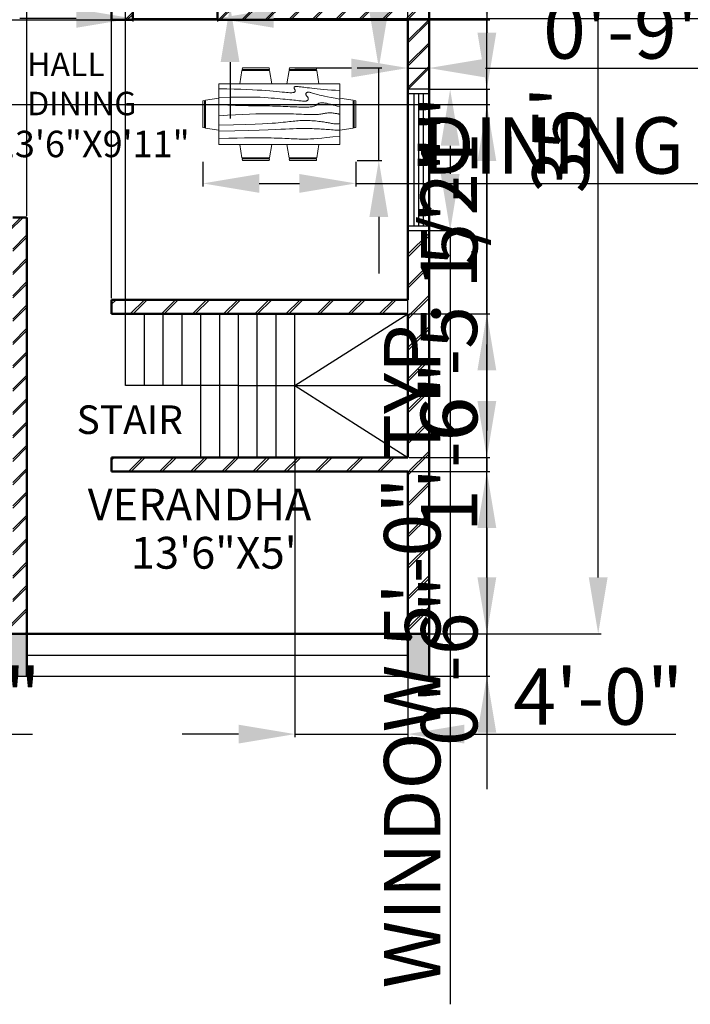
# Model space of a CAD drawing. Units: inches. Extents: x -584 to 444, y 228 to 1001.
# Tile 3 of 5: x -68 to 217, y 228 to 647. Entities that reach past the tile are written whole.
import ezdxf

# ---------------------------------------------------------------- set-up
doc = ezdxf.new("R2010")
doc.units = ezdxf.units.IN
for name, color, linetype, lineweight in [('A-ANNO-DIMS', 2, 'Continuous', 18), ('A-AREA-IDEN', 7, 'Continuous', 25), ('A-FLOR-STRS', 7, 'Continuous', 25), ('A-FURN', 8, 'Continuous', 18), ('A-GLAZ', 4, 'Continuous', 25), ('A-WALL', 7, 'Continuous', 50), ('A-WALL-PATT', 3, 'Continuous', 13)]:
    doc.layers.add(name, color=color, linetype=linetype, lineweight=lineweight)
doc.styles.get("Standard").update_dxf_attribs({"font": 'arial.ttf'})
doc.dimstyles.new('ISO-25', dxfattribs={"dimtxt": 24, "dimasz": 24, "dimexe": 1.25, "dimexo": 0.625, "dimtad": 1, "dimdec": 1, "dimlunit": 3, "dimtxsty": 'Standard', "dimcen": 2.5, "dimadec": 0, "dimazin": 0, "dimtfac": 1, "dimtdec": 1, "dimtmove": 0, "dimatfit": 3, "dimfxl": 1, "dimarcsym": 0})

# ---------------------------------------------------------------- blocks, each defined once
blk = doc.blocks.new('Dining Set - 36 x 72 in.')
for p, q in [((-22.2343, 26.00059), (-23.4847, 17.99762)), ((-22.2304, 26), (-5.7608, 26)), ((-22, 27.5), (-22.1562, 26.50042)), ((-5.8416, 26.5), (-22.1534, 26.5)), ((-22, 27.5), (-6, 27.5)), ((-5.8437, 26.49966), (-6, 27.5)), ((-4.5152, 17.99762), (-5.7655, 25.99926)), ((5.7657, 26.00059), (4.5153, 17.99762)), ((5.7696, 26), (22.2392, 26)), ((6, 27.5), (5.8438, 26.50042)), ((22.1584, 26.5), (5.8466, 26.5)), ((6, 27.5), (22, 27.5)), ((22.1563, 26.49966), (22, 27.5)), ((23.4848, 17.99762), (22.2345, 25.99926)), ((36, 18), (-36, 18)), ((-36, 18), (-36, -18)), ((36, -18), (36, 18)), ((-45.5, 8), (-44.5004, 8.15617)), ((-45.5, 8), (-45.5, -8)), ((-44.5, -8.15843), (-44.5, 8.15338)), ((-44.0006, 8.23428), (-35.9976, 9.48474)), ((-44, 8.23041), (-44, -8.23915)), ((44.0006, 8.23428), (35.9976, 9.48474)), ((44, 8.23041), (44, -8.23915)), ((44.5, -8.15843), (44.5, 8.15338)), ((45.5, 8), (44.5005, 8.15617)), ((45.5, 8), (45.5, -8)), ((-44.4997, -8.15631), (-45.5, -8)), ((-35.9976, -9.48476), (-43.9993, -8.2345)), ((35.9976, -9.48476), (43.9993, -8.2345)), ((44.4997, -8.15631), (45.5, -8)), ((-36, -18), (36, -18)), ((-22.2343, -26.0006), (-23.4847, -17.99762)), ((-4.5152, -17.99762), (-5.7655, -25.99928)), ((5.7657, -26.0006), (4.5153, -17.99762)), ((23.4848, -17.99762), (22.2345, -25.99928)), ((-22.2304, -26), (-5.7608, -26)), ((-22, -27.5), (-22.1562, -26.50044)), ((-5.8416, -26.5), (-22.1534, -26.5)), ((-22, -27.5), (-6, -27.5)), ((-5.8437, -26.49967), (-6, -27.5)), ((5.7696, -26), (22.2392, -26)), ((6, -27.5), (5.8438, -26.50044)), ((22.1584, -26.5), (5.8466, -26.5)), ((6, -27.5), (22, -27.5)), ((22.1563, -26.49967), (22, -27.5))]:
    blk.add_line(p, q)
for points in [[(-36, 15), (-31.1772, 14.97754), (-26.8079, 14.91406), (-22.8538, 14.81543), (-19.276, 14.6875), (-16.0362, 14.53613), (-13.0957, 14.36718), (-10.4159, 14.18652), (-7.9583, 14), (-5.6904, 13.81315), (-3.6035, 13.63021), (-1.6954, 13.45508), (0.0365, 13.29166), (1.5945, 13.14388), (2.9811, 13.01562), (4.1988, 12.9108), (5.25, 12.83333), (6.1393, 12.78613), (6.8802, 12.76823), (7.4883, 12.77767), (7.9792, 12.8125), (8.3685, 12.87077), (8.6719, 12.95052), (8.9049, 13.0498), (9.0833, 13.16666), (9.2205, 13.29899), (9.3216, 13.44401), (9.3895, 13.59879), (9.4271, 13.76041), (9.4373, 13.92594), (9.4232, 14.09245), (9.3875, 14.257), (9.3333, 14.41666), (9.2638, 14.56917), (9.1836, 14.71484), (9.0975, 14.85465), (9.0104, 14.98958), (8.9272, 15.1206), (8.8529, 15.2487), (8.7922, 15.37483), (8.75, 15.5), (8.7305, 15.62467), (8.7344, 15.74739), (8.7617, 15.86621), (8.8125, 15.97916), (8.8867, 16.08431), (8.9844, 16.17968), (9.1055, 16.26334), (9.25, 16.33333), (9.4189, 16.38802), (9.6172, 16.42708), (9.8506, 16.45052), (10.125, 16.45833), (10.4463, 16.45052), (10.8203, 16.42708), (11.2529, 16.38802), (11.75, 16.33333), (12.3184, 16.26318), (12.9694, 16.17838), (13.7151, 16.07991), (14.5677, 15.96875), (15.5395, 15.84586), (16.6426, 15.71224), (17.8893, 15.56884), (19.2917, 15.41666), (20.859, 15.25667), (22.5879, 15.08984), (24.4721, 14.91715), (26.5052, 14.73958), (28.6809, 14.5581), (30.9929, 14.3737), (33.4347, 14.18733), (36, 14)], [(-36, 10), (-28.9766, 10.14274), (-23.1725, 10.20442), (-18.4241, 10.19775), (-14.5677, 10.13541), (-11.4399, 10.03011), (-8.877, 9.89453), (-6.7154, 9.74137), (-4.7917, 9.58333), (-2.9698, 9.43082), (-1.2246, 9.28515), (0.4415, 9.14534), (2.026, 9.01041), (3.5266, 8.87939), (4.9408, 8.7513), (6.266, 8.62516), (7.5, 8.5), (8.6411, 8.37549), (9.6914, 8.2539), (10.6538, 8.13818), (11.5312, 8.03125), (12.3267, 7.93603), (13.043, 7.85547), (13.6831, 7.79248), (14.25, 7.75), (14.7471, 7.7303), (15.1797, 7.73307), (15.5537, 7.75732), (15.875, 7.80208), (16.1494, 7.86637), (16.3828, 7.94922), (16.5811, 8.04964), (16.75, 8.16666), (16.8944, 8.29915), (17.0143, 8.44531), (17.1089, 8.60319), (17.1771, 8.77083), (17.218, 8.94629), (17.2305, 9.1276), (17.2137, 9.31282), (17.1667, 9.5), (17.0895, 9.6875), (16.987, 9.875), (16.8649, 10.0625), (16.7292, 10.25), (16.5856, 10.4375), (16.4401, 10.625), (16.2985, 10.8125), (16.1667, 11), (16.05, 11.18733), (15.9518, 11.3737), (15.8752, 11.5581), (15.8229, 11.73958), (15.798, 11.91715), (15.8034, 12.08984), (15.842, 12.25667), (15.9167, 12.41666), (16.0295, 12.56836), (16.1784, 12.70833), (16.3605, 12.83268), (16.5729, 12.9375), (16.8127, 13.01888), (17.0768, 13.07291), (17.3625, 13.0957), (17.6667, 13.08333), (17.9894, 13.03312), (18.3418, 12.94726), (18.7382, 12.82918), (19.1927, 12.68229), (19.7195, 12.51001), (20.3327, 12.31575), (21.0465, 12.10294), (21.875, 11.875), (22.8357, 11.63354), (23.959, 11.37304), (25.2786, 11.08618), (26.8282, 10.76562), (28.6414, 10.40405), (30.752, 9.99414), (33.1936, 9.52856), (36, 9)], [(-36, 5.5), (-30.7157, 5.3348), (-26.069, 5.20963), (-21.9946, 5.11767), (-18.4271, 5.05208), (-15.3009, 5.00602), (-12.5508, 4.97265), (-10.1112, 4.94515), (-7.9167, 4.91666), (-5.909, 4.88167), (-4.0586, 4.83984), (-2.3429, 4.79215), (-0.7396, 4.73958), (0.7739, 4.6831), (2.22, 4.6237), (3.6213, 4.56233), (5, 4.5), (6.373, 4.43782), (7.7344, 4.3776), (9.0723, 4.32129), (10.375, 4.27083), (11.6309, 4.22819), (12.8281, 4.19531), (13.9551, 4.17415), (15, 4.16666), (15.954, 4.17448), (16.819, 4.19791), (17.6001, 4.23698), (18.3021, 4.29166), (18.9299, 4.36198), (19.4883, 4.44791), (19.9823, 4.54948), (20.4167, 4.66666), (20.7969, 4.79899), (21.1302, 4.94401), (21.4245, 5.09879), (21.6875, 5.26041), (21.9271, 5.42594), (22.1511, 5.59245), (22.3672, 5.757), (22.5834, 5.91666), (22.8065, 6.06868), (23.0404, 6.21093), (23.2879, 6.34147), (23.5521, 6.45833), (23.8358, 6.55957), (24.142, 6.64323), (24.4735, 6.70735), (24.8334, 6.75), (25.2235, 6.76969), (25.642, 6.76692), (26.0858, 6.74267), (26.5521, 6.69791), (27.0379, 6.63362), (27.5404, 6.55078), (28.0565, 6.45036), (28.5834, 6.33333), (29.1242, 6.19987), (29.7071, 6.04687), (30.3661, 5.87044), (31.1354, 5.66666), (32.0493, 5.43164), (33.142, 5.16146), (34.4475, 4.85221), (36, 4.5)], [(-36, -1), (-30.7915, -0.6591), (-26.0195, -0.38216), (-21.6519, -0.16284), (-17.6563, 0.00521), (-14.0005, 0.12833), (-10.6523, 0.21289), (-7.5796, 0.26522), (-4.75, 0.29166), (-2.134, 0.29793), (0.2878, 0.28711), (2.5317, 0.26163), (4.6146, 0.22396), (6.5529, 0.17651), (8.3633, 0.12174), (10.0623, 0.06209), (11.6667, 0), (13.1899, -0.06201), (14.6341, -0.1211), (15.9982, -0.17432), (17.2813, -0.21875), (18.4823, -0.25147), (19.6003, -0.26953), (20.6343, -0.27002), (21.5834, -0.25), (22.4481, -0.20768), (23.2357, -0.14584), (23.9549, -0.06836), (24.6146, 0.02083), (25.2235, 0.11784), (25.7904, 0.21875), (26.3241, 0.31966), (26.8334, 0.41666), (27.3265, 0.50618), (27.8099, 0.58593), (28.2894, 0.65397), (28.7709, 0.70833), (29.2601, 0.74707), (29.763, 0.76823), (30.2855, 0.76985), (30.8334, 0.75), (31.4088, 0.70784), (31.9994, 0.64713), (32.589, 0.57275), (33.1615, 0.48958), (33.7008, 0.4025), (34.1908, 0.3164), (34.6153, 0.23616), (34.9584, 0.16666), (35.2099, 0.11165), (35.3848, 0.07031), (35.504, 0.04069), (35.5886, 0.02083), (35.6594, 0.00879), (35.7377, 0.0026), (35.8442, 0.00032), (36, 0)], [(-36, -6.5), (-27.1843, -6.31267), (-20.084, -6.1263), (-14.469, -5.9419), (-10.1094, -5.76042), (-6.7752, -5.58285), (-4.2363, -5.41016), (-2.2629, -5.24333), (-0.625, -5.08334), (0.8708, -4.93099), (2.2715, -4.78646), (3.5872, -4.64974), (4.8281, -4.52084), (6.0046, -4.39974), (7.127, -4.28646), (8.2053, -4.18099), (9.25, -4.08334), (10.2705, -3.99382), (11.2734, -3.91407), (12.2647, -3.84603), (13.25, -3.79167), (14.2354, -3.75293), (15.2266, -3.73177), (16.2295, -3.73015), (17.25, -3.75), (18.2912, -3.79248), (19.3451, -3.85547), (20.4009, -3.93604), (21.4479, -4.03125), (22.4754, -4.13819), (23.4727, -4.25391), (24.4289, -4.37549), (25.3334, -4.5), (26.1785, -4.62492), (26.9694, -4.74935), (27.7145, -4.87281), (28.4219, -4.99479), (29.1, -5.11483), (29.7572, -5.23242), (30.4016, -5.34709), (31.0417, -5.45834), (31.6837, -5.56437), (32.3262, -5.65821), (32.9658, -5.73153), (33.599, -5.77604), (34.2224, -5.78345), (34.8327, -5.74545), (35.4264, -5.65373), (36, -5.5)], [(-36, -10), (-26.4022, -9.81299), (-18.4675, -9.62891), (-11.9839, -9.45069), (-6.7396, -9.28125), (-2.5226, -9.12354), (0.8789, -8.98047), (3.6769, -8.85498), (6.0833, -8.75), (8.2767, -8.66765), (10.3021, -8.60677), (12.1712, -8.56543), (13.8958, -8.54167), (15.4876, -8.53353), (16.9583, -8.53907), (18.3197, -8.55632), (19.5834, -8.58334), (20.7616, -8.61841), (21.8685, -8.66081), (22.9188, -8.71004), (23.9271, -8.76563), (24.9081, -8.82707), (25.8763, -8.89388), (26.8465, -8.96558), (27.8334, -9.04167), (28.8474, -9.12118), (29.8828, -9.20117), (30.93, -9.27824), (31.9792, -9.34896), (33.0205, -9.40991), (34.0443, -9.45768), (35.0407, -9.48885), (36, -9.5)], [(-36, -14.5), (-30.0881, -14.33513), (-25.0332, -14.21224), (-20.7312, -14.12647), (-17.0781, -14.07292), (-13.97, -14.04671), (-11.3027, -14.04297), (-8.9724, -14.05681), (-6.875, -14.08334), (-4.9224, -14.11833), (-3.0905, -14.16016), (-1.3709, -14.20785), (0.2448, -14.26042), (1.7647, -14.3169), (3.1973, -14.3763), (4.5507, -14.43767), (5.8333, -14.5), (7.0554, -14.5621), (8.235, -14.62175), (9.3922, -14.67652), (10.5469, -14.72396), (11.7192, -14.76164), (12.929, -14.78711), (14.1965, -14.79794), (15.5417, -14.79167), (16.9933, -14.76424), (18.6152, -14.70508), (20.4804, -14.60197), (22.6615, -14.44271), (25.2312, -14.21509), (28.2624, -13.9069), (31.8277, -13.50594), (36, -13)]]:
    blk.add_lwpolyline(points)
blk = doc.blocks.new('*D7')
at = {"layer": 'A-ANNO-DIMS', "color": 0, "lineweight": -2, "transparency": 16777216}
for p, q in [((106.48, 805.54), (179.05, 805.54)), ((177.8, 409.54), (177.8, 781.54)), ((106.48, 385.54), (179.05, 385.54))]:
    blk.add_line(p, q, dxfattribs=at)
at = {"layer": 'A-ANNO-DIMS', "color": 0, "transparency": 16777216}
for points in [[(173.8, 781.54), (181.8, 781.54), (177.8, 805.54)], [(173.8, 409.54), (181.8, 409.54), (177.8, 385.54)]]:
    blk.add_solid(points, dxfattribs=at)
at = {"layer": 'Defpoints', "color": 0, "transparency": 16777216}
for p in [(105.86, 805.54), (177.8, 805.54), (105.86, 385.54)]:
    blk.add_point(p, dxfattribs=at)
at = {"layer": 'A-ANNO-DIMS', "color": 0, "transparency": 16777216, "insert": (164.91, 595.54), "char_height": 24, "attachment_point": 5, "rotation": 90}
blk.add_mtext("35'", dxfattribs=at)
blk = doc.blocks.new('WIN-60IN')
for p, q in [((60, 9), (0, 9)), ((0, 9), (0, 0)), ((2, 9), (2, 0)), ((58, 0), (58, 9)), ((60, 0), (60, 9)), ((2, 6.5), (58, 6.5)), ((2, 4.5), (58, 4.5)), ((0, 0), (60, 0)), ((2, 2.5), (58, 2.5))]:
    blk.add_line(p, q)
blk = doc.blocks.new('*D11')
at = {"layer": 'A-ANNO-DIMS', "color": 0, "lineweight": -2, "transparency": 16777216}
for p, q in [((106.48, 617.04), (116.11, 617.04)), ((114.86, 593.04), (114.86, 581.04)), ((106.48, 557.04), (116.11, 557.04)), ((114.86, 557.04), (114.86, 228.09))]:
    blk.add_line(p, q, dxfattribs=at)
at = {"layer": 'A-ANNO-DIMS', "color": 0, "transparency": 16777216}
for points in [[(110.86, 593.04), (118.86, 593.04), (114.86, 617.04)], [(110.86, 581.04), (118.86, 581.04), (114.86, 557.04)]]:
    blk.add_solid(points, dxfattribs=at)
at = {"layer": 'Defpoints', "color": 0, "transparency": 16777216}
for p in [(105.86, 617.04), (105.86, 557.04), (114.86, 557.04)]:
    blk.add_point(p, dxfattribs=at)
at = {"layer": 'A-ANNO-DIMS', "color": 0, "transparency": 16777216, "insert": (101.81, 380.56), "char_height": 24, "attachment_point": 5, "rotation": 90}
blk.add_mtext('WINDOW 5\'-0" TYP.', dxfattribs=at)
blk = doc.blocks.new('*D12')
at = {"layer": 'A-ANNO-DIMS', "color": 0, "lineweight": -2, "transparency": 16777216}
for p, q in [((72.86, 626.04), (48.86, 626.04)), ((96.86, 617.66), (96.86, 627.29)), ((96.86, 626.04), (105.86, 626.04)), ((105.86, 617.66), (105.86, 627.29)), ((129.86, 626.04), (301.4, 626.04))]:
    blk.add_line(p, q, dxfattribs=at)
at = {"layer": 'A-ANNO-DIMS', "color": 0, "transparency": 16777216}
for points in [[(72.86, 630.04), (72.86, 622.04), (96.86, 626.04)], [(129.86, 630.04), (129.86, 622.04), (105.86, 626.04)]]:
    blk.add_solid(points, dxfattribs=at)
at = {"layer": 'Defpoints', "color": 0, "transparency": 16777216}
for p in [(105.86, 626.04), (96.86, 617.04), (105.86, 617.04)]:
    blk.add_point(p, dxfattribs=at)
at = {"layer": 'A-ANNO-DIMS', "color": 0, "transparency": 16777216, "insert": (227.63, 638.92), "char_height": 24, "attachment_point": 5}
blk.add_mtext('0\'-9" TYP.', dxfattribs=at)
blk = doc.blocks.new('*D17')
at = {"layer": 'A-ANNO-DIMS', "color": 0, "lineweight": -2, "transparency": 16777216}
for p, q in [((-20.14, 651.91), (-20.14, 645.89)), ((15.86, 651.91), (15.86, 645.89)), ((-44.14, 647.14), (-68.14, 647.14)), ((-20.14, 647.14), (15.86, 647.14)), ((39.86, 647.14), (444.11, 647.14))]:
    blk.add_line(p, q, dxfattribs=at)
at = {"layer": 'A-ANNO-DIMS', "color": 0, "transparency": 16777216}
for points in [[(-44.14, 651.14), (-44.14, 643.14), (-20.14, 647.14)], [(39.86, 651.14), (39.86, 643.14), (15.86, 647.14)]]:
    blk.add_solid(points, dxfattribs=at)
at = {"layer": 'Defpoints', "color": 0, "transparency": 16777216}
for p in [(-20.14, 652.54), (15.86, 652.54), (15.86, 647.14)]:
    blk.add_point(p, dxfattribs=at)
at = {"layer": 'A-ANNO-DIMS', "color": 0, "transparency": 16777216, "insert": (253.99, 660.19), "char_height": 24, "attachment_point": 5}
blk.add_mtext('SWING DOOR 3\'-0" TYP.', dxfattribs=at)
blk = doc.blocks.new('*D18')
at = {"layer": 'A-ANNO-DIMS', "color": 0, "lineweight": -2, "transparency": 16777216}
for p, q in [((21.26, 712.54), (21.26, 884.06)), ((16.48, 688.54), (22.51, 688.54)), ((21.26, 652.54), (21.26, 688.54)), ((16.48, 652.54), (22.51, 652.54)), ((21.26, 628.54), (21.26, 604.54))]:
    blk.add_line(p, q, dxfattribs=at)
at = {"layer": 'A-ANNO-DIMS', "color": 0, "transparency": 16777216}
for points in [[(17.26, 712.54), (25.26, 712.54), (21.26, 688.54)], [(17.26, 628.54), (25.26, 628.54), (21.26, 652.54)]]:
    blk.add_solid(points, dxfattribs=at)
at = {"layer": 'Defpoints', "color": 0, "transparency": 16777216}
for p in [(15.86, 688.54), (21.26, 688.54), (15.86, 652.54)]:
    blk.add_point(p, dxfattribs=at)
at = {"layer": 'A-ANNO-DIMS', "color": 0, "transparency": 16777216, "insert": (8.37, 810.3), "char_height": 24, "attachment_point": 5, "rotation": 90}
blk.add_mtext('3\'-0" TYP.', dxfattribs=at)
blk = doc.blocks.new('*D25')
at = {"layer": 'A-ANNO-DIMS', "color": 0, "lineweight": -2, "transparency": 16777216}
for p, q in [((9.69, 586.14), (9.69, 575.76)), ((74.75, 586.14), (74.75, 575.76)), ((33.69, 577.01), (50.75, 577.01)), ((74.75, 577.01), (363.79, 577.01))]:
    blk.add_line(p, q, dxfattribs=at)
at = {"layer": 'A-ANNO-DIMS', "color": 0, "transparency": 16777216}
for points in [[(33.69, 581.01), (33.69, 573.01), (9.69, 577.01)], [(50.75, 581.01), (50.75, 573.01), (74.75, 577.01)]]:
    blk.add_solid(points, dxfattribs=at)
at = {"layer": 'Defpoints', "color": 0, "transparency": 16777216}
for p in [(9.69, 586.77), (74.75, 586.77), (74.75, 577.01)]:
    blk.add_point(p, dxfattribs=at)
at = {"layer": 'A-ANNO-DIMS', "color": 0, "transparency": 16777216, "insert": (231.27, 590.04), "char_height": 24, "attachment_point": 5}
blk.add_mtext('DINING SET 5\'-5"', dxfattribs=at)
blk = doc.blocks.new('*D26')
at = {"layer": 'A-ANNO-DIMS', "color": 0, "lineweight": -2, "transparency": 16777216}
for p, q in [((84.51, 650.09), (84.51, 795.05)), ((75.37, 626.09), (85.76, 626.09)), ((84.51, 586.77), (84.51, 626.09)), ((75.37, 586.77), (85.76, 586.77)), ((84.51, 562.77), (84.51, 538.77))]:
    blk.add_line(p, q, dxfattribs=at)
at = {"layer": 'A-ANNO-DIMS', "color": 0, "transparency": 16777216}
for points in [[(80.51, 650.09), (88.51, 650.09), (84.51, 626.09)], [(80.51, 562.77), (88.51, 562.77), (84.51, 586.77)]]:
    blk.add_solid(points, dxfattribs=at)
at = {"layer": 'Defpoints', "color": 0, "transparency": 16777216}
for p in [(74.75, 626.09), (84.51, 626.09), (74.75, 586.77)]:
    blk.add_point(p, dxfattribs=at)
at = {"layer": 'A-ANNO-DIMS', "color": 0, "transparency": 16777216, "insert": (71.46, 734.57), "char_height": 24, "attachment_point": 5, "rotation": 90}
blk.add_mtext('3\'-3 1/2"', dxfattribs=at)
blk = doc.blocks.new('*D27')
at = {"layer": 'A-ANNO-DIMS', "color": 0, "lineweight": -2, "transparency": 16777216}
for p, q in [((130.46, 409.54), (130.46, 496.33)), ((106.48, 385.54), (131.71, 385.54)), ((130.46, 367.54), (130.46, 385.54)), ((106.48, 367.54), (131.71, 367.54)), ((130.46, 343.54), (130.46, 319.54))]:
    blk.add_line(p, q, dxfattribs=at)
at = {"layer": 'A-ANNO-DIMS', "color": 0, "transparency": 16777216}
for points in [[(126.46, 409.54), (134.46, 409.54), (130.46, 385.54)], [(126.46, 343.54), (134.46, 343.54), (130.46, 367.54)]]:
    blk.add_solid(points, dxfattribs=at)
at = {"layer": 'Defpoints', "color": 0, "transparency": 16777216}
for p in [(105.86, 385.54), (130.46, 385.54), (105.86, 367.54)]:
    blk.add_point(p, dxfattribs=at)
at = {"layer": 'A-ANNO-DIMS', "color": 0, "transparency": 16777216, "insert": (117.58, 464.93), "char_height": 24, "attachment_point": 5, "rotation": 90}
blk.add_mtext('1\'-6"', dxfattribs=at)
blk = doc.blocks.new('*D29')
at = {"layer": 'A-ANNO-DIMS', "color": 0, "lineweight": -2, "transparency": 16777216}
for p, q in [((-209.14, 795.91), (-209.14, 341.69)), ((-176.14, 795.91), (-176.14, 341.69)), ((-233.14, 342.94), (-257.14, 342.94)), ((-209.14, 342.94), (-176.14, 342.94)), ((-152.14, 342.94), (-62.69, 342.94))]:
    blk.add_line(p, q, dxfattribs=at)
at = {"layer": 'A-ANNO-DIMS', "color": 0, "transparency": 16777216}
for points in [[(-233.14, 346.94), (-233.14, 338.94), (-209.14, 342.94)], [(-152.14, 346.94), (-152.14, 338.94), (-176.14, 342.94)]]:
    blk.add_solid(points, dxfattribs=at)
at = {"layer": 'Defpoints', "color": 0, "transparency": 16777216}
for p in [(-209.14, 796.54), (-176.14, 796.54), (-176.14, 342.94)]:
    blk.add_point(p, dxfattribs=at)
at = {"layer": 'A-ANNO-DIMS', "color": 0, "transparency": 16777216, "insert": (-95.41, 355.82), "char_height": 24, "attachment_point": 5}
blk.add_mtext('2\'-9"', dxfattribs=at)
blk = doc.blocks.new('*D32')
at = {"layer": 'A-ANNO-DIMS', "color": 0, "lineweight": -2, "transparency": 16777216}
for p, q in [((106.48, 694.54), (131.71, 694.54)), ((130.46, 670.54), (130.46, 641.04)), ((106.48, 617.04), (131.71, 617.04)), ((130.46, 617.04), (130.46, 471.93))]:
    blk.add_line(p, q, dxfattribs=at)
at = {"layer": 'A-ANNO-DIMS', "color": 0, "transparency": 16777216}
for points in [[(126.46, 670.54), (134.46, 670.54), (130.46, 694.54)], [(126.46, 641.04), (134.46, 641.04), (130.46, 617.04)]]:
    blk.add_solid(points, dxfattribs=at)
at = {"layer": 'Defpoints', "color": 0, "transparency": 16777216}
for p in [(105.86, 694.54), (105.86, 617.04), (130.46, 617.04)]:
    blk.add_point(p, dxfattribs=at)
at = {"layer": 'A-ANNO-DIMS', "color": 0, "transparency": 16777216, "insert": (117.42, 532.49), "char_height": 24, "attachment_point": 5, "rotation": 90}
blk.add_mtext('6\'-5 1/2"', dxfattribs=at)
blk = doc.blocks.new('*D35')
at = {"layer": 'A-ANNO-DIMS', "color": 0, "lineweight": -2, "transparency": 16777216}
for p, q in [((130.46, 484.54), (130.46, 508.54)), ((97.48, 460.54), (131.71, 460.54)), ((130.46, 460.54), (130.46, 454.54)), ((97.48, 454.54), (131.71, 454.54)), ((130.46, 430.54), (130.46, 341.49))]:
    blk.add_line(p, q, dxfattribs=at)
at = {"layer": 'A-ANNO-DIMS', "color": 0, "transparency": 16777216}
for points in [[(126.46, 484.54), (134.46, 484.54), (130.46, 460.54)], [(126.46, 430.54), (134.46, 430.54), (130.46, 454.54)]]:
    blk.add_solid(points, dxfattribs=at)
at = {"layer": 'Defpoints', "color": 0, "transparency": 16777216}
for p in [(96.86, 460.54), (96.86, 454.54), (130.46, 454.54)]:
    blk.add_point(p, dxfattribs=at)
at = {"layer": 'A-ANNO-DIMS', "color": 0, "transparency": 16777216, "insert": (117.58, 374.01), "char_height": 24, "attachment_point": 5, "rotation": 90}
blk.add_mtext('0\'-6"', dxfattribs=at)
blk = doc.blocks.new('*D36')
at = {"layer": 'A-ANNO-DIMS', "color": 0, "lineweight": -2, "transparency": 16777216}
for p, q in [((-23.14, 522.16), (-23.14, 831.39)), ((0.86, 830.14), (72.86, 830.14)), ((96.86, 522.16), (96.86, 831.39))]:
    blk.add_line(p, q, dxfattribs=at)
at = {"layer": 'A-ANNO-DIMS', "color": 0, "transparency": 16777216}
for points in [[(0.86, 834.14), (0.86, 826.14), (-23.14, 830.14)], [(72.86, 834.14), (72.86, 826.14), (96.86, 830.14)]]:
    blk.add_solid(points, dxfattribs=at)
at = {"layer": 'Defpoints', "color": 0, "transparency": 16777216}
for p in [(96.86, 830.14), (-23.14, 521.54), (96.86, 521.54)]:
    blk.add_point(p, dxfattribs=at)
at = {"layer": 'A-ANNO-DIMS', "color": 0, "transparency": 16777216, "insert": (36.86, 843.02), "char_height": 24, "attachment_point": 5}
blk.add_mtext('10\'-0"', dxfattribs=at)
blk = doc.blocks.new('*D37')
at = {"layer": 'A-ANNO-DIMS', "color": 0, "lineweight": -2, "transparency": 16777216}
for p, q in [((48.86, 459.91), (48.86, 341.69)), ((96.86, 453.91), (96.86, 341.69)), ((24.86, 342.94), (0.86, 342.94)), ((48.86, 342.94), (96.86, 342.94)), ((120.86, 342.94), (210.87, 342.94))]:
    blk.add_line(p, q, dxfattribs=at)
at = {"layer": 'A-ANNO-DIMS', "color": 0, "transparency": 16777216}
for points in [[(24.86, 346.94), (24.86, 338.94), (48.86, 342.94)], [(120.86, 346.94), (120.86, 338.94), (96.86, 342.94)]]:
    blk.add_solid(points, dxfattribs=at)
at = {"layer": 'Defpoints', "color": 0, "transparency": 16777216}
for p in [(48.86, 460.54), (96.86, 454.54), (96.86, 342.94)]:
    blk.add_point(p, dxfattribs=at)
at = {"layer": 'A-ANNO-DIMS', "color": 0, "transparency": 16777216, "insert": (177.86, 355.82), "char_height": 24, "attachment_point": 5}
blk.add_mtext('4\'-0"', dxfattribs=at)
blk = doc.blocks.new('*D38')
at = {"layer": 'A-ANNO-DIMS', "color": 0, "lineweight": -2, "transparency": 16777216}
for p, q in [((130.46, 521.54), (130.46, 610.59)), ((97.48, 521.54), (131.71, 521.54)), ((130.46, 484.54), (130.46, 497.54)), ((97.48, 460.54), (131.71, 460.54))]:
    blk.add_line(p, q, dxfattribs=at)
at = {"layer": 'A-ANNO-DIMS', "color": 0, "transparency": 16777216}
for points in [[(126.46, 497.54), (134.46, 497.54), (130.46, 521.54)], [(126.46, 484.54), (134.46, 484.54), (130.46, 460.54)]]:
    blk.add_solid(points, dxfattribs=at)
at = {"layer": 'Defpoints', "color": 0, "transparency": 16777216}
for p in [(96.86, 521.54), (130.46, 521.54), (96.86, 460.54)]:
    blk.add_point(p, dxfattribs=at)
at = {"layer": 'A-ANNO-DIMS', "color": 0, "transparency": 16777216, "insert": (117.58, 578.06), "char_height": 24, "attachment_point": 5, "rotation": 90}
blk.add_mtext('5\'-1"', dxfattribs=at)
blk = doc.blocks.new('*D40')
at = {"layer": 'A-ANNO-DIMS', "color": 0, "lineweight": -2, "transparency": 16777216}
for p, q in [((130.46, 670.54), (130.46, 759.57)), ((-76.52, 646.54), (131.71, 646.54)), ((130.46, 610.54), (130.46, 646.54)), ((-116.52, 610.54), (131.71, 610.54)), ((130.46, 586.54), (130.46, 562.54))]:
    blk.add_line(p, q, dxfattribs=at)
at = {"layer": 'A-ANNO-DIMS', "color": 0, "transparency": 16777216}
for points in [[(126.46, 670.54), (134.46, 670.54), (130.46, 646.54)], [(126.46, 586.54), (134.46, 586.54), (130.46, 610.54)]]:
    blk.add_solid(points, dxfattribs=at)
at = {"layer": 'Defpoints', "color": 0, "transparency": 16777216}
for p in [(-77.14, 646.54), (130.46, 646.54), (-117.14, 610.54)]:
    blk.add_point(p, dxfattribs=at)
at = {"layer": 'A-ANNO-DIMS', "color": 0, "transparency": 16777216, "insert": (117.57, 727.05), "char_height": 24, "attachment_point": 5, "rotation": 90}
blk.add_mtext('3\'-0"', dxfattribs=at)
blk = doc.blocks.new('*D41')
at = {"layer": 'A-ANNO-DIMS', "color": 0, "lineweight": -2, "transparency": 16777216}
for p, q in [((-89.14, 830.14), (-113.14, 830.14)), ((-65.14, 563.16), (-65.14, 831.39)), ((-65.14, 830.14), (-29.14, 830.14)), ((-29.14, 528.16), (-29.14, 831.39)), ((-5.14, 830.14), (83.89, 830.14))]:
    blk.add_line(p, q, dxfattribs=at)
at = {"layer": 'A-ANNO-DIMS', "color": 0, "transparency": 16777216}
for points in [[(-89.14, 834.14), (-89.14, 826.14), (-65.14, 830.14)], [(-5.14, 834.14), (-5.14, 826.14), (-29.14, 830.14)]]:
    blk.add_solid(points, dxfattribs=at)
at = {"layer": 'Defpoints', "color": 0, "transparency": 16777216}
for p in [(-29.14, 830.14), (-65.14, 562.54), (-29.14, 527.54)]:
    blk.add_point(p, dxfattribs=at)
at = {"layer": 'A-ANNO-DIMS', "color": 0, "transparency": 16777216, "insert": (51.37, 843.02), "char_height": 24, "attachment_point": 5}
blk.add_mtext('3\'-0"', dxfattribs=at)

msp = doc.modelspace()

# ---------------------------------------------------------------- hatches: boundary and pattern name
at = {"layer": 'A-WALL-PATT'}
h = msp.add_hatch(dxfattribs=at)
h.set_pattern_fill('JIS_LC_8A', color=256, scale=0.9)
h.set_pattern_definition([(45, (105.857, 805.537), (-4.96389, 4.96389), []), (45, (106.757, 805.537), (-4.96389, 4.96389), [])])
h.paths.add_polyline_path([(105.86, 694.54), (96.86, 694.54), (96.86, 652.54), (15.86, 652.54), (15.86, 646.54), (96.86, 646.54), (96.86, 617.04), (105.86, 617.04)])
h.paths.add_polyline_path([(-77.14, 655.54), (-83.14, 655.54), (-83.14, 652.54), (-209.14, 652.54), (-209.14, 796.54), (-176.14, 796.54), (-176.14, 805.54), (-218.14, 805.54), (-218.14, 610.54), (-209.14, 610.54), (-209.14, 646.54), (-77.14, 646.54)])
h.paths.add_polyline_path([(-209.14, 598.54), (-218.14, 598.54), (-218.14, 505.54), (-209.14, 505.54), (-209.14, 556.54), (-111.14, 556.54), (-110.14, 556.54), (-110.14, 562.54), (-111.14, 562.54), (-111.14, 610.54), (-117.14, 610.54), (-117.14, 562.54), (-209.14, 562.54)])
h.paths.add_polyline_path([(-59.14, 805.54), (-116.14, 805.54), (-116.14, 796.54), (-83.14, 796.54), (-83.14, 691.54), (-77.14, 691.54), (-77.14, 796.54), (-59.14, 796.54)])
h.paths.add_polyline_path([(105.86, 805.54), (-47.14, 805.54), (-47.14, 796.54), (-29.14, 796.54), (-29.14, 712.54), (-47.14, 712.54), (-47.14, 706.54), (-29.14, 706.54), (-29.14, 646.54), (-20.14, 646.54), (-20.14, 652.54), (-23.14, 652.54), (-23.14, 796.54), (96.86, 796.54), (96.86, 754.54), (105.86, 754.54)])
h.paths.add_polyline_path([(-65.14, 385.54), (-65.14, 562.54), (-71.14, 562.54), (-74.14, 562.54), (-74.14, 556.54), (-71.14, 556.54), (-71.14, 394.54), (-209.14, 394.54), (-209.14, 445.54), (-218.14, 445.54), (-218.14, 385.54)])
h = msp.add_hatch(dxfattribs=at)
h.set_pattern_fill('JIS_LC_8A', color=256, scale=1.2)
h.paths.add_polyline_path([(105.86, 557.04), (96.86, 557.04), (96.86, 527.54), (-29.14, 527.54), (-29.14, 521.54), (96.86, 521.54), (96.86, 460.54), (-29.14, 460.54), (-29.14, 454.54), (96.86, 454.54), (96.86, 394.54), (96.86, 385.54), (105.86, 385.54)])
h = msp.add_hatch(dxfattribs=at)
h.set_pattern_fill('BRICK', color=256, scale=0.2)
h.paths.add_polyline_path([(-65.14, 385.54), (-74.14, 385.54), (-74.14, 367.54), (-65.14, 367.54)])
h.paths.add_polyline_path([(105.86, 385.54), (96.86, 385.54), (96.86, 367.54), (105.86, 367.54)])

# ---------------------------------------------------------------- linework, layer by layer
at = {"layer": 'A-FLOR-STRS'}
for p, q in [((-23.14, 491.04), (-23.14, 521.54)), ((-15.14, 491.04), (-15.14, 521.54)), ((-7.14, 491.04), (-7.14, 521.54)), ((0.86, 491.04), (0.86, 521.54)), ((8.86, 460.54), (8.86, 521.54)), ((16.86, 460.54), (16.86, 521.54)), ((24.86, 460.54), (24.86, 521.54)), ((32.86, 460.54), (32.86, 521.54)), ((40.86, 460.54), (40.86, 521.54)), ((48.86, 460.54), (48.86, 521.54)), ((48.86, 491.04), (96.86, 521.54)), ((24.86, 491.04), (-23.14, 491.04)), ((24.86, 491.04), (96.86, 491.04)), ((48.86, 491.04), (96.86, 460.54)), ((-65.14, 376.54), (96.86, 376.54)), ((-74.14, 367.54), (105.86, 367.54))]:
    msp.add_line(p, q, dxfattribs=at)
at = {"layer": 'A-WALL'}
for p, q in [((105.86, 385.54), (105.86, 805.54)), ((-29.14, 706.54), (-29.14, 646.54)), ((-20.14, 652.54), (-20.14, 646.54)), ((15.86, 652.54), (15.86, 646.54)), ((-20.14, 646.54), (-29.14, 646.54)), ((96.86, 646.54), (15.86, 646.54)), ((96.86, 527.54), (96.86, 646.54)), ((-71.14, 562.54), (-65.14, 562.54)), ((-65.14, 556.54), (-65.14, 562.54)), ((-65.14, 556.54), (-65.14, 394.54)), ((96.86, 527.54), (-29.14, 527.54)), ((-29.14, 527.54), (-29.14, 521.54)), ((96.86, 521.54), (-29.14, 521.54)), ((96.86, 460.54), (96.86, 521.54)), ((-29.14, 460.54), (-29.14, 454.54)), ((-29.14, 460.54), (96.86, 460.54)), ((-29.14, 454.54), (96.86, 454.54)), ((96.86, 394.54), (96.86, 454.54)), ((-65.14, 394.54), (-65.14, 367.54)), ((96.86, 394.54), (96.86, 385.54)), ((-218.14, 385.54), (105.86, 385.54)), ((96.86, 367.54), (96.86, 385.54)), ((105.86, 367.54), (105.86, 385.54))]:
    msp.add_line(p, q, dxfattribs=at)

# ---------------------------------------------------------------- block references
at = {"layer": 'A-FURN', "xscale": 0.7149745617862227, "yscale": 0.7149745617862227, "zscale": 0.7149745617862227}
msp.add_blockref('Dining Set - 36 x 72 in.', (42.22, 606.43), dxfattribs=at)
at = {"layer": 'A-GLAZ', "rotation": 270.0000000000002}
msp.add_blockref('WIN-60IN', (96.86, 617.04), dxfattribs=at)

# ---------------------------------------------------------------- texts
at = {"layer": 'A-AREA-IDEN', "attachment_point": 1}
for s, width, gutter_width, insert, char_height in [('HALL\\PDINING', 576.7965, 49.9, (-65, 632.59), 9.98), ('13\'6"X9\'11"', 648.8713, 56.13, (-78.72, 599.38), 11.2267), ('STAIR', 701.2838, 60.67, (-44, 482.64), 12.134), ('VERANDHA ', 781.4857, 67.61, (-39.27, 447.32), 13.521), ('13\'6"X5\'', 781.4857, 67.61, (-20.9, 426.76), 13.521)]:
    msp.add_mtext_dynamic_manual_height_columns(s, width=width, gutter_width=gutter_width, heights=[0], dxfattribs=dict(at, insert=insert, char_height=char_height))

# ---------------------------------------------------------------- dimensions: what is measured, and where the dimension line sits
at = {"layer": 'A-ANNO-DIMS'}
for base, p1, p2, angle, text, picture, middle in [((21.26, 688.54), (15.86, 652.54), (15.86, 688.54), 90, '<> TYP.', '*D18', (8.37, 810.3)), ((114.86, 557.04), (105.86, 617.04), (105.86, 557.04), 270, 'WINDOW <> TYP.', '*D11', (101.81, 380.56))]:
    dim = msp.add_linear_dim(base=base, p1=p1, p2=p2, angle=angle, text=text, dimstyle='ISO-25', override={"dimdec": 1, "dimlfac": 1, "dimrnd": 0, "dimzin": 1, "dimdsep": 46, "dimlunit": 4, "dimfrac": 2}, dxfattribs=at)
    dim.commit()
    dim.dimension.update_dxf_attribs({"geometry": picture, "text_midpoint": middle})
for base, p1, p2, picture, middle in [((-29.14, 830.14), (-65.14, 562.54), (-29.14, 527.54), '*D41', (51.37, 843.02)), ((96.86, 830.14), (-23.14, 521.54), (96.86, 521.54), '*D36', (36.86, 843.02)), ((-176.14, 342.94), (-209.14, 796.54), (-176.14, 796.54), '*D29', (-95.41, 355.82)), ((96.86, 342.94), (48.86, 460.54), (96.86, 454.54), '*D37', (177.86, 355.82))]:
    dim = msp.add_linear_dim(base=base, p1=p1, p2=p2, dimstyle='ISO-25', override={"dimdec": 1, "dimlfac": 1, "dimrnd": 0, "dimzin": 1, "dimdsep": 46, "dimlunit": 4, "dimfrac": 2}, dxfattribs=at)
    dim.commit()
    dim.dimension.update_dxf_attribs({"geometry": picture, "text_midpoint": middle})
for base, p1, p2, override, picture, middle in [((177.8, 805.54), (105.86, 385.54), (105.86, 805.54), {"dimclrd": 0, "dimclre": 0, "dimclrt": 0}, '*D7', (164.91, 595.54)), ((84.51, 626.09), (74.75, 586.77), (74.75, 626.09), {"dimdec": 1, "dimlfac": 1, "dimrnd": 0, "dimzin": 1, "dimdsep": 46, "dimlunit": 4, "dimfrac": 2}, '*D26', (71.46, 734.57)), ((130.46, 646.54), (-117.14, 610.54), (-77.14, 646.54), {"dimdec": 1, "dimlfac": 1, "dimrnd": 0, "dimzin": 1, "dimdsep": 46, "dimlunit": 4, "dimfrac": 2}, '*D40', (117.57, 727.05)), ((130.46, 617.04), (105.86, 694.54), (105.86, 617.04), {"dimdec": 1, "dimlfac": 1, "dimrnd": 0, "dimzin": 1, "dimdsep": 46, "dimlunit": 4, "dimfrac": 2}, '*D32', (117.42, 532.49)), ((130.46, 521.54), (96.86, 460.54), (96.86, 521.54), {"dimdec": 1, "dimlfac": 1, "dimrnd": 0, "dimzin": 1, "dimdsep": 46, "dimlunit": 4, "dimfrac": 2}, '*D38', (117.58, 578.06)), ((130.46, 454.54), (96.86, 460.54), (96.86, 454.54), {"dimdec": 1, "dimlfac": 1, "dimrnd": 0, "dimzin": 1, "dimdsep": 46, "dimlunit": 4, "dimfrac": 2}, '*D35', (117.58, 374.01)), ((130.46, 385.54), (105.86, 367.54), (105.86, 385.54), {"dimdec": 1, "dimlfac": 1, "dimrnd": 0, "dimzin": 1, "dimdsep": 46, "dimlunit": 4, "dimfrac": 2}, '*D27', (117.58, 464.93))]:
    dim = msp.add_linear_dim(base=base, p1=p1, p2=p2, angle=90, dimstyle='ISO-25', override=override, dxfattribs=at)
    dim.commit()
    dim.dimension.update_dxf_attribs({"geometry": picture, "text_midpoint": middle})
for base, p1, p2, text, picture, middle in [((15.86, 647.14), (-20.14, 652.54), (15.86, 652.54), 'SWING DOOR <> TYP.', '*D17', (253.99, 660.19)), ((105.86, 626.04), (96.86, 617.04), (105.86, 617.04), '<> TYP.', '*D12', (227.63, 638.92)), ((74.75, 577.01), (9.69, 586.77), (74.75, 586.77), 'DINING SET <>', '*D25', (231.27, 590.04))]:
    dim = msp.add_linear_dim(base=base, p1=p1, p2=p2, text=text, dimstyle='ISO-25', override={"dimdec": 1, "dimlfac": 1, "dimrnd": 0, "dimzin": 1, "dimdsep": 46, "dimlunit": 4, "dimfrac": 2}, dxfattribs=at)
    dim.commit()
    dim.dimension.update_dxf_attribs({"geometry": picture, "text_midpoint": middle})

doc.saveas('drawing.dxf')
